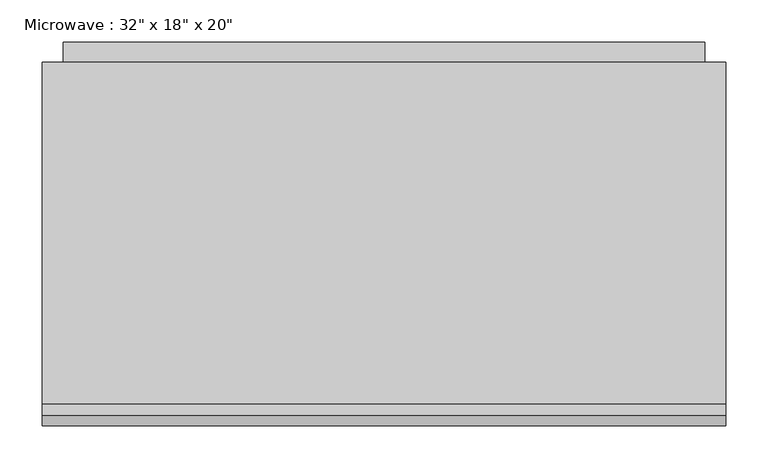
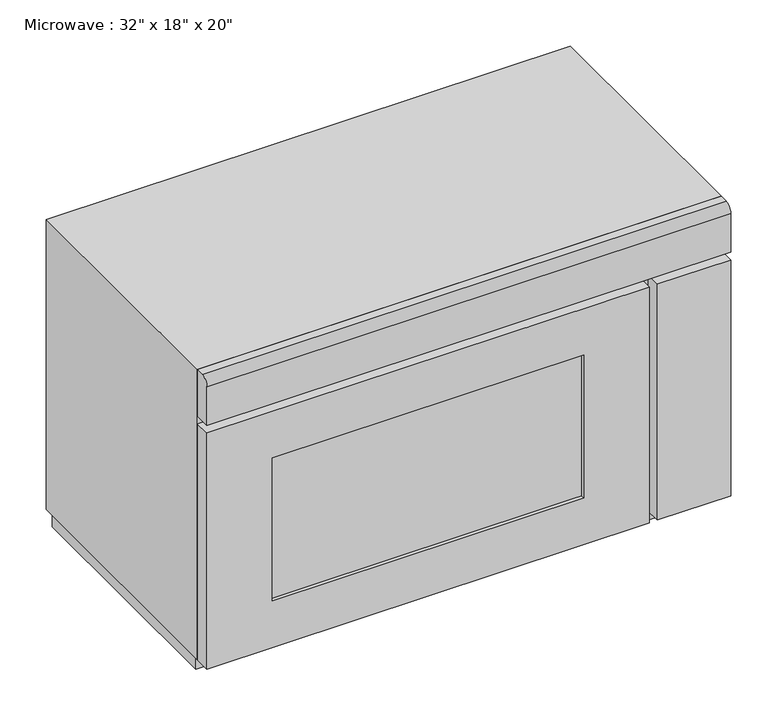
"""IFC4 building model written with IfcOpenShell, lengths in millimetres: proxy geometry."""

from ifc_helpers import new_model, si_unit, point, frame, frame_2d, origin, place, context, project, spatial, polyline, circle_curve, trimmed, segment, composite_curve, outline, extrude, faceted_brep, source, transform, mapped, element, save


def proxy_5fdb4fb0(model_context):
    return source(origin(), model_context, "Body", "SolidModel", [
        extrude(outline(polyline([(678.4897523, -575.3305058), (195.4928773, -575.3305058), (195.4928773, -568.9805058), (678.4897523, -568.9805058), (678.4897523, -575.3305058)])), frame((0.0, 0.0, 1022.35), z_axis=(0.0, 0.0, 1.0), x_axis=(1.0, 0.0, 0.0)), (0.0, 0.0, 1.0), 234.95),
        extrude(outline(polyline([(1333.5, 780.0897523), (1333.5, 93.8928773), (946.15, 93.8928773), (946.15, 780.0897523), (1333.5, 780.0897523)]), holes=[polyline([(1257.3, 678.4897523), (1022.35, 678.4897523), (1022.35, 195.4928773), (1257.3, 195.4928773), (1257.3, 678.4897523)])]), frame((0.0, -581.6805058, 0.0), z_axis=(0.0, 1.0, 0.0), x_axis=(0.0, 0.0, 1.0)), (0.0, 0.0, 1.0), 25.4),
        extrude(outline(polyline([(906.6928773, -581.6805058), (792.7897523, -581.6805058), (792.7897523, -556.2805058), (906.6928773, -556.2805058), (906.6928773, -581.6805058)])), frame((0.0, 0.0, 946.15), z_axis=(0.0, 0.0, 1.0), x_axis=(1.0, 0.0, 0.0)), (0.0, 0.0, 1.0), 387.35),
        extrude(outline(composite_curve([segment(polyline([(-568.9805058, 1422.4), (-556.2805058, 1422.4), (-556.2805058, 1346.2), (-581.6805058, 1346.2), (-581.6805058, 1409.7)]), True, "CONTINUOUS"), segment(trimmed(circle_curve(frame_2d((-568.9805058, 1409.7)), 12.7), [point((-581.6805058, 1409.7))], [point((-568.9805058, 1422.4))], False, "CARTESIAN"), True, "CONTINUOUS")], self_intersect=False)), frame((93.8928773, 0.0, 0.0), z_axis=(1.0, 0.0, 0.0), x_axis=(0.0, 1.0, 0.0)), (0.0, 0.0, 1.0), 812.8),
        extrude(outline(polyline([(-125.6441495, 1397.0), (-125.6441495, 961.946551), (-151.0441495, 936.546551), (-151.0441495, 1397.0), (-125.6441495, 1397.0)])), frame((119.2928773, 0.0, 0.0), z_axis=(1.0, 0.0, 0.0), x_axis=(0.0, 1.0, 0.0)), (0.0, 0.0, 1.0), 762.0),
        faceted_brep([(906.6928773, -149.8805058, 1422.4), (93.8928773, -149.8805058, 1422.4), (93.8928773, -556.2805058, 1422.4), (906.6928773, -556.2805058, 1422.4), (906.6928773, -149.8805058, 946.15), (906.6928773, -556.2805058, 946.15), (93.8928773, -556.2805058, 946.15), (93.8928773, -149.8805058, 946.15), (849.9397523, -556.2805058, 1271.0014904), (849.9397523, -556.2805058, 1020.1764904), (150.6460023, -556.2805058, 1020.1764904), (150.6460023, -556.2805058, 1271.0014904), (849.9397523, -226.0805058, 1271.0014904), (150.6460023, -226.0805058, 1271.0014904), (150.6460023, -226.0805058, 1020.1764904), (849.9397523, -226.0805058, 1020.1764904)], [[[0, 1, 2, 3]], [[4, 5, 6, 7]], [[1, 0, 4, 7]], [[2, 1, 7, 6]], [[3, 2, 6, 5], [8, 9, 10, 11]], [[0, 3, 5, 4]], [[12, 13, 14, 15]], [[12, 15, 9, 8]], [[15, 14, 10, 9]], [[14, 13, 11, 10]], [[13, 12, 8, 11]]]),
        extrude(outline(polyline([(897.1678773, -149.8805058), (897.1678773, -535.6430058), (103.4178773, -535.6430058), (103.4178773, -149.8805058), (897.1678773, -149.8805058)])), frame((0.0, 0.0, 914.4), z_axis=(0.0, 0.0, 1.0), x_axis=(1.0, 0.0, 0.0)), (0.0, 0.0, 1.0), 31.75),
    ])


if __name__ == "__main__":
    model = new_model("IFC4")
    model_context = context("Model", 3, world=origin())
    ifc_project = project(units=[si_unit("LENGTHUNIT", "METRE", prefix="MILLI")], contexts=[model_context])
    site = spatial("IfcSite", under=ifc_project)
    building = spatial("IfcBuilding", under=site)
    placement = place(None, origin())
    proxy_shape = proxy_5fdb4fb0(model_context)
    element("IfcBuildingElementProxy", 1, Name="Microwave : 32\" x 18\" x 20\"", ObjectType="Microwave : 32\" x 18\" x 20\"", at=placement, inside=building, context=model_context, shape_type="MappedRepresentation", body=[
        mapped(proxy_shape, transform((0.0, 0.0, 0.0), x_axis=(1.0, 0.0, 0.0), y_axis=(0.0, 1.0, 0.0), z_axis=(0.0, 0.0, 1.0))),
    ])
    save(model, "model.ifc")

# Revit data of these elements
# Type "Microwave : 32\" x 18\" x 20\""
#   Assembly Code = "E1090400"
#   Depth = 1' - 6"
#   Height = 1' - 8"
#   Width = 2' - 8"
#   Microwave Material = Laminate, Ivory, Matte
#   Default Elevation = 0
# Element 1 (IfcBuildingElementProxy, "Microwave : 32\" x 18\" x 20\"")
#   Materials on its faces: "Laminate, Ivory, Matte", "Glass"
# Materials
#   "Laminate, Ivory, Matte": class "Plastic", colour RGB 247 247 239, transparency 0, Description = "Plastic Laminate - Ivory, Matte", Cost = 0
#   "Glass": class "Glass", colour RGB 0 128 192, transparency 0.75, Description = "Soda Lime Glass", Cost = 0
